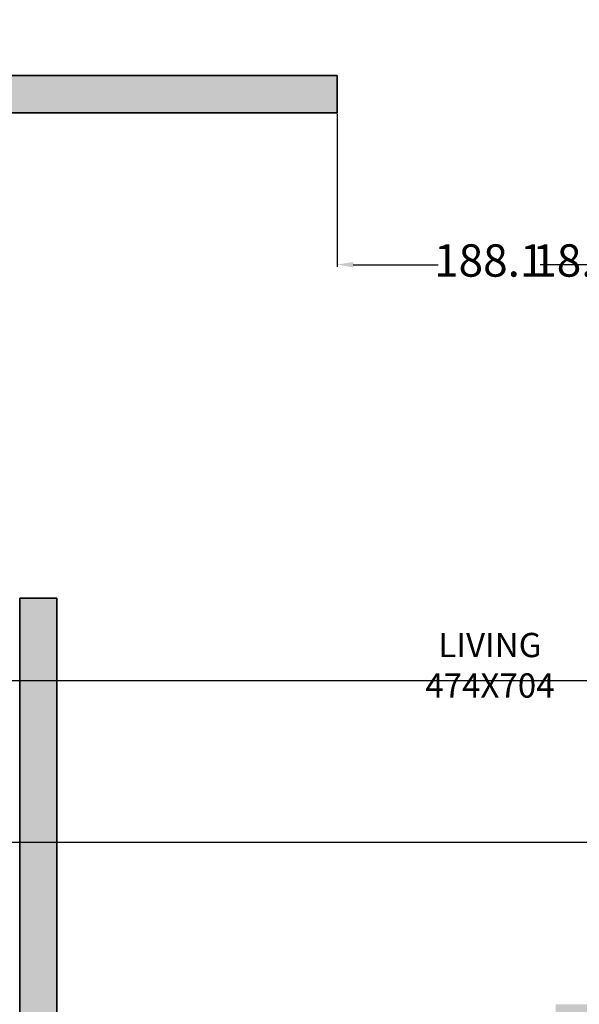
# Model space of a CAD drawing. Units: centimetres. Extents: x 2137 to 3697, y 183 to 2094.
# Tile 4 of 8: x 2685 to 3031, y 600 to 1208. Entities that reach past the tile are written whole.
import ezdxf

# ---------------------------------------------------------------- set-up
doc = ezdxf.new("R2010")
doc.units = ezdxf.units.CM
for name, color, linetype, lineweight in [('A-ANNO-DIMS', 2, 'Continuous', 18), ('A-AREA-IDEN', 7, 'Continuous', 25), ('A-WALL', 7, 'Continuous', 35), ('A-WALL-PATT', 52, 'Continuous', 13)]:
    doc.layers.add(name, color=color, linetype=linetype, lineweight=lineweight)
doc.styles.get("Standard").update_dxf_attribs({"font": 'arial.ttf'})
doc.dimstyles.new('ISO-25', dxfattribs={"dimtxt": 20, "dimasz": 10, "dimexe": 1.25, "dimexo": 0.625, "dimtad": 0, "dimtxsty": 'Standard', "dimcen": 2.5, "dimadec": 0, "dimazin": 0, "dimtfac": 1, "dimtmove": 0, "dimatfit": 3, "dimfxl": 1, "dimarcsym": 0})

# ---------------------------------------------------------------- blocks, each defined once
blk = doc.blocks.new('*D38')
at = {"layer": 'A-ANNO-DIMS', "color": 0, "lineweight": -2, "transparency": 16777216}
for p, q in [((2857.4, 1986.58), (2174.92, 1986.58)), ((2176.17, 1976.58), (2176.17, 1171.09)), ((2176.17, 306.58), (2176.17, 1112.07)), ((2269.4, 296.58), (2174.92, 296.58))]:
    blk.add_line(p, q, dxfattribs=at)
at = {"layer": 'A-ANNO-DIMS', "color": 0, "transparency": 16777216}
for points in [[(2174.51, 1976.58), (2177.84, 1976.58), (2176.17, 1986.58)], [(2174.51, 306.58), (2177.84, 306.58), (2176.17, 296.58)]]:
    blk.add_solid(points, dxfattribs=at)
at = {"layer": 'Defpoints', "color": 0, "transparency": 16777216}
for p in [(2176.17, 1986.58), (2858.02, 1986.58), (2270.02, 296.58)]:
    blk.add_point(p, dxfattribs=at)
at = {"layer": 'A-ANNO-DIMS', "color": 0, "transparency": 16777216, "insert": (2176.17, 1141.58), "char_height": 20, "attachment_point": 5, "rotation": 90}
blk.add_mtext('1690', dxfattribs=at)
blk = doc.blocks.new('*D42')
at = {"layer": 'A-ANNO-DIMS', "color": 0, "lineweight": -2, "transparency": 16777216}
for p, q in [((3183.4, 799.58), (2174.92, 799.58)), ((2176.17, 789.58), (2176.17, 771.32)), ((2176.17, 709.58), (2176.17, 727.84)), ((3183.4, 699.58), (2174.92, 699.58))]:
    blk.add_line(p, q, dxfattribs=at)
at = {"layer": 'A-ANNO-DIMS', "color": 0, "transparency": 16777216}
for points in [[(2174.51, 789.58), (2177.84, 789.58), (2176.17, 799.58)], [(2174.51, 709.58), (2177.84, 709.58), (2176.17, 699.58)]]:
    blk.add_solid(points, dxfattribs=at)
at = {"layer": 'Defpoints', "color": 0, "transparency": 16777216}
for p in [(2176.17, 799.58), (3184.02, 799.58), (3184.02, 699.58)]:
    blk.add_point(p, dxfattribs=at)
at = {"layer": 'A-ANNO-DIMS', "color": 0, "transparency": 16777216, "insert": (2176.17, 749.58), "char_height": 20, "attachment_point": 5, "rotation": 90}
blk.add_mtext('100', dxfattribs=at)
blk = doc.blocks.new('*D64')
at = {"layer": 'A-ANNO-DIMS', "color": 0, "lineweight": -2, "transparency": 16777216}
for p, q in [((2881.02, 1149.95), (2881.02, 1055.48)), ((3069.12, 1149.95), (3069.12, 1055.48)), ((2891.02, 1056.73), (2943.57, 1056.73)), ((3059.12, 1056.73), (3006.57, 1056.73))]:
    blk.add_line(p, q, dxfattribs=at)
at = {"layer": 'A-ANNO-DIMS', "color": 0, "transparency": 16777216}
for points in [[(2891.02, 1058.4), (2891.02, 1055.06), (2881.02, 1056.73)], [(3059.12, 1058.4), (3059.12, 1055.06), (3069.12, 1056.73)]]:
    blk.add_solid(points, dxfattribs=at)
at = {"layer": 'Defpoints', "color": 0, "transparency": 16777216}
for p in [(2881.02, 1150.58), (3069.12, 1150.58), (2881.02, 1056.73)]:
    blk.add_point(p, dxfattribs=at)
at = {"layer": 'A-ANNO-DIMS', "color": 0, "transparency": 16777216, "insert": (2975.07, 1056.73), "char_height": 20, "attachment_point": 5}
blk.add_mtext('188.1', dxfattribs=at)
blk = doc.blocks.new('*D65')
at = {"layer": 'A-ANNO-DIMS', "color": 0, "lineweight": -2, "transparency": 16777216}
for p, q in [((3089.12, 1149.95), (3089.12, 1055.48)), ((3107.59, 1149.95), (3107.59, 1055.48)), ((3079.12, 1056.73), (3069.12, 1056.73)), ((3107.59, 1056.73), (3089.12, 1056.73)), ((3117.59, 1056.73), (3127.59, 1056.73))]:
    blk.add_line(p, q, dxfattribs=at)
at = {"layer": 'A-ANNO-DIMS', "color": 0, "transparency": 16777216}
for points in [[(3079.12, 1058.4), (3079.12, 1055.06), (3089.12, 1056.73)], [(3117.59, 1058.4), (3117.59, 1055.06), (3107.59, 1056.73)]]:
    blk.add_solid(points, dxfattribs=at)
at = {"layer": 'Defpoints', "color": 0, "transparency": 16777216}
for p in [(3089.12, 1150.58), (3107.59, 1150.58), (3089.12, 1056.73)]:
    blk.add_point(p, dxfattribs=at)
at = {"layer": 'A-ANNO-DIMS', "color": 0, "transparency": 16777216, "insert": (3035.69, 1056.73), "char_height": 20, "attachment_point": 5}
blk.add_mtext('18.47', dxfattribs=at)

msp = doc.modelspace()

# ---------------------------------------------------------------- hatches: boundary and pattern name
at = {"layer": 'A-WALL-PATT'}
h = msp.add_hatch(color=256, dxfattribs=at)
h.dxf.hatch_style = 1
h.paths.add_polyline_path([(2413.023, 1526.579), (2270.023, 1526.579), (2270.023, 1413.579), (2293.023, 1413.579), (2293.023, 1503.579), (2413.023, 1503.579)])
h.paths.add_polyline_path([(2744.523, 1526.579), (2563.023, 1526.579), (2563.023, 1503.579), (2638.023, 1503.579), (2683.023, 1503.579), (2683.023, 1296.579), (2706.023, 1296.579), (2706.023, 1503.579), (2744.523, 1503.579)])
h.paths.add_polyline_path([(2881.023, 1541.602), (2858.023, 1541.602), (2858.023, 1526.579), (2819.523, 1526.579), (2819.523, 1503.579), (2858.023, 1503.579), (2858.023, 1311.579), (2781.023, 1311.579), (2781.023, 1296.579), (2858.023, 1296.579), (2858.023, 1273.579), (2881.023, 1273.579)])
h.paths.add_polyline_path([(3207.023, 1745.579), (2881.023, 1745.579), (2881.023, 1963.579), (2913.523, 1963.579), (2913.523, 1986.579), (2858.023, 1986.579), (2858.023, 1691.602), (2881.023, 1691.602), (2881.023, 1722.579), (3184.023, 1722.579), (3184.023, 1321.579), (3207.023, 1321.579)])
h.paths.add_polyline_path([(3072.523, 1986.579), (2988.523, 1986.579), (2988.523, 1963.579), (3021.023, 1963.579), (3021.023, 1820.579), (3036.023, 1820.579), (3036.023, 1963.579), (3072.523, 1963.579)], flags=17)
h.paths.add_polyline_path([(3207.023, 1986.579), (3147.523, 1986.579), (3147.523, 1963.579), (3184.023, 1963.579), (3184.023, 1845.579), (3207.023, 1845.579)], flags=17)
h.paths.add_polyline_path([(3590.023, 1986.579), (3307.023, 1986.579), (3307.023, 1963.579), (3567.023, 1963.579), (3567.023, 1888.579), (3590.023, 1888.579), (3590.023, 1963.579)])
h.paths.add_polyline_path([(3590.023, 1738.579), (3567.023, 1738.579), (3567.023, 1663.579), (3372.023, 1663.579), (3372.023, 1648.579), (3567.023, 1648.579), (3567.023, 1514.579), (3387.023, 1514.579), (3387.023, 1573.579), (3372.023, 1573.579), (3372.023, 1514.579), (3307.023, 1514.579), (3307.023, 1491.579), (3567.023, 1491.579), (3567.023, 1431.579), (3590.023, 1431.579)])
h.paths.add_polyline_path([(3590.023, 1281.579), (3567.023, 1281.579), (3567.023, 1221.579), (3184.023, 1221.579), (3184.023, 922.579), (3207.023, 922.579), (3207.023, 1198.579), (3567.023, 1198.579), (3567.023, 1055.075), (3590.023, 1055.075)])
h.paths.add_polyline_path([(3590.023, 905.075), (3567.023, 905.075), (3567.023, 774.852), (3590.023, 774.852)])
h.paths.add_polyline_path([(3590.023, 624.852), (3567.023, 624.852), (3567.023, 599.579), (3184.023, 599.579), (3184.023, 576.579), (3590.023, 576.579)])
h.paths.add_polyline_path([(3590.023, 443.579), (3567.023, 443.579), (3567.023, 420.579), (3590.023, 420.579)])
h.paths.add_polyline_path([(3225.908, 443.579), (3202.908, 443.579), (3202.908, 420.579), (3225.908, 420.579)])
h.paths.add_polyline_path([(3039.023, 599.579), (3016.023, 599.579), (3016.023, 443.579), (2937.023, 443.579), (2937.023, 420.579), (3039.023, 420.579)])
h.paths.add_polyline_path([(2787.023, 443.579), (2708.023, 443.579), (2708.023, 850.579), (2685.023, 850.579), (2685.023, 319.579), (2564.023, 319.579), (2564.023, 296.579), (2708.023, 296.579), (2708.023, 420.579), (2787.023, 420.579)])
h.paths.add_polyline_path([(2414.023, 319.579), (2293.023, 319.579), (2293.023, 412.079), (2270.023, 412.079), (2270.023, 296.579), (2414.023, 296.579)])
h.paths.add_polyline_path([(2592.023, 677.579), (2293.023, 677.579), (2293.023, 715.079), (2270.023, 715.079), (2270.023, 562.079), (2293.023, 562.079), (2293.023, 637.079), (2293.023, 654.579), (2592.023, 654.579)])
h.paths.add_polyline_path([(2592.023, 850.579), (2526.773, 850.579), (2526.441, 850.508), (2377.032, 850.508), (2293.023, 850.579), (2293.023, 925.579), (2270.023, 925.579), (2270.023, 790.079), (2293.023, 790.079), (2293.023, 827.579), (2569.023, 827.579), (2569.023, 752.579), (2592.023, 752.579)])
h.paths.add_polyline_path([(2293.023, 1263.579), (2270.023, 1263.579), (2270.023, 1075.579), (2293.023, 1075.579), (2293.023, 1150.579), (2881.023, 1150.579), (2881.023, 1173.579), (2293.023, 1173.579)])

# ---------------------------------------------------------------- linework, layer by layer
at = {"layer": 'A-WALL'}
for p, q in [((2293.023, 1173.579), (2881.023, 1173.579)), ((2881.023, 1173.579), (2881.023, 1150.579)), ((2293.023, 1150.579), (2881.023, 1150.579)), ((2685.023, 850.579), (2685.023, 319.579)), ((2708.023, 850.579), (2685.023, 850.579)), ((2708.023, 850.579), (2708.023, 443.579))]:
    msp.add_line(p, q, dxfattribs=at)

# ---------------------------------------------------------------- texts
at = {"layer": 'A-AREA-IDEN', "insert": (2951.007, 829.152), "char_height": 15, "attachment_point": 1}
msp.add_mtext_dynamic_manual_height_columns('\\pxqc;LIVING\\P474X704', width=48.94887, gutter_width=12.5, heights=[0], dxfattribs=at)

# ---------------------------------------------------------------- dimensions: what is measured, and where the dimension line sits
at = {"layer": 'A-ANNO-DIMS'}
for base, p1, p2, angle, override, picture, middle in [((2176.173, 1986.579), (2270.023, 296.579), (2858.023, 1986.579), 90, {"dimdec": 0, "dimlfac": 1, "dimrnd": 0, "dimzin": 0, "dimdsep": 46, "dimlunit": 2}, '*D38', (2176.173, 1141.579)), ((2881.023, 1056.729), (3069.116, 1150.579), (2881.023, 1150.579), 180, {"dimdec": 1, "dimlfac": 1, "dimrnd": 0, "dimzin": 0, "dimdsep": 46, "dimlunit": 2}, '*D64', (2975.069, 1056.729)), ((3089.116, 1056.729), (3107.587, 1150.579), (3089.116, 1150.579), 180, {"dimdec": 2, "dimlfac": 1, "dimrnd": 0, "dimzin": 0, "dimdsep": 46, "dimlunit": 2}, '*D65', (3035.687, 1056.729)), ((2176.173, 799.579), (3184.023, 699.579), (3184.023, 799.579), 90, {"dimdec": 0, "dimlfac": 1, "dimrnd": 0, "dimzin": 0, "dimdsep": 46, "dimlunit": 2}, '*D42', (2176.173, 749.579))]:
    dim = msp.add_linear_dim(base=base, p1=p1, p2=p2, angle=angle, dimstyle='ISO-25', override=override, dxfattribs=at)
    dim.commit()
    dim.dimension.update_dxf_attribs({"geometry": picture, "text_midpoint": middle})

doc.saveas('drawing.dxf')
